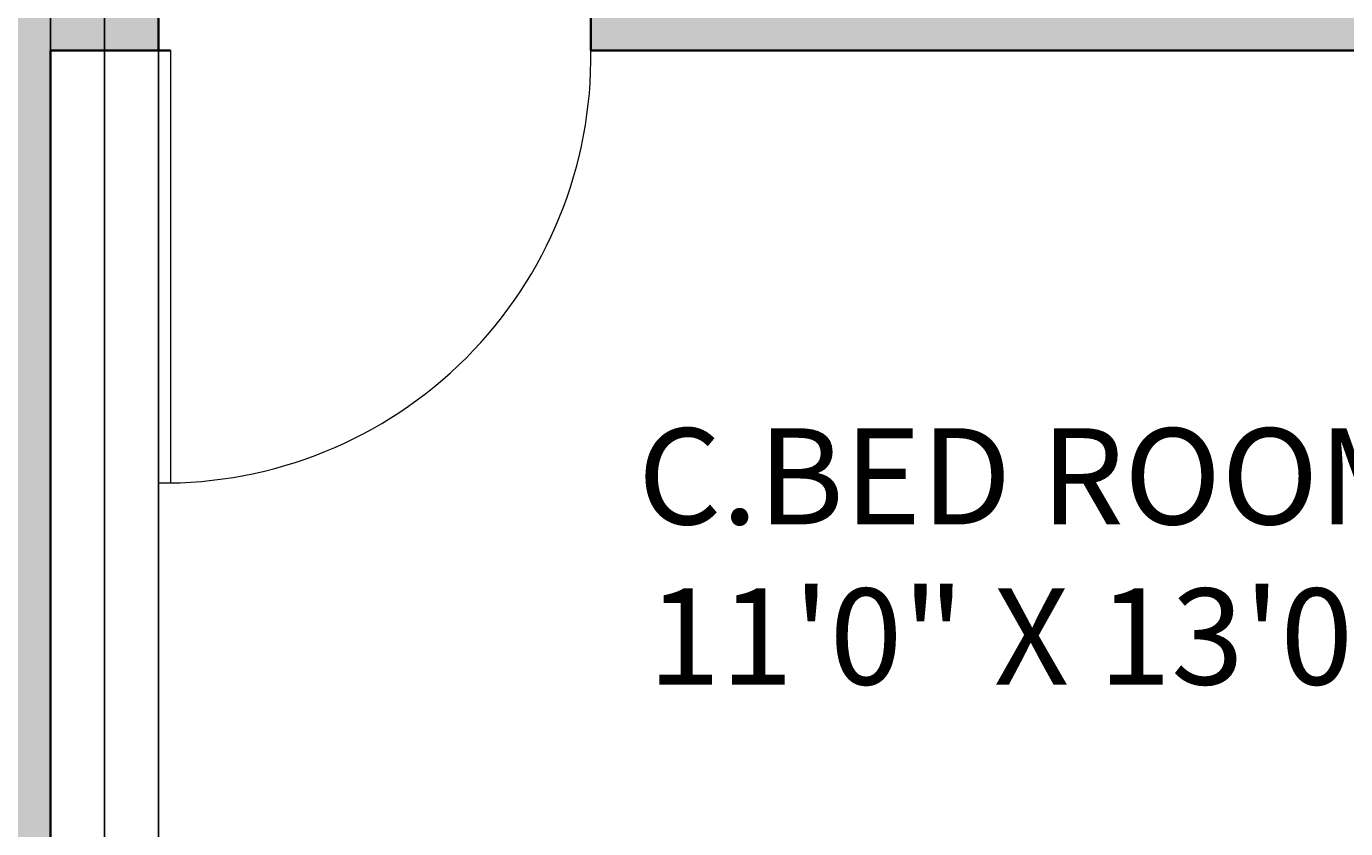
# Model space of a CAD drawing. Units: inches. Extents: x 1567 to 1964, y 1813 to 2447.
# Tile 5 of 28: x 1797 to 1907, y 2059 to 2125. Entities that reach past the tile are written whole.
import ezdxf

# ---------------------------------------------------------------- set-up
doc = ezdxf.new("R2010")
doc.units = ezdxf.units.IN
for name, color, linetype, lineweight in [('A-ANNO-DIMS', 2, 'Continuous', 18), ('A-AREA-IDEN', 7, 'Continuous', 18), ('A-DOOR', 4, 'Continuous', 18), ('A-WALL', 7, 'Continuous', 35)]:
    doc.layers.add(name, color=color, linetype=linetype, lineweight=lineweight)
doc.layers.add('A-FURN-PATT', color=252, linetype='Continuous', lineweight=13, true_color=0x939598)
doc.layers.add('A-WALL-PATT', color=251, linetype='Continuous', lineweight=13, true_color=0x636466)
doc.styles.get("Standard").update_dxf_attribs({"font": 'arial.ttf'})
doc.dimstyles.get("Standard").update_dxf_attribs({"dimtxt": 0.18, "dimasz": 0.18, "dimexe": 0.18, "dimexo": 0.0625, "dimgap": 0.09, "dimtad": 0, "dimtih": 1, "dimtoh": 1, "dimdec": 4, "dimzin": 0, "dimdsep": 46, "dimtxsty": 'Standard', "dimcen": 0.09, "dimadec": 0, "dimazin": 0, "dimtfac": 1, "dimtdec": 4, "dimtofl": 0, "dimtmove": 0, "dimatfit": 3, "dimfxl": 1, "dimtolj": 1, "dimtzin": 0, "dimarcsym": 0})

# ---------------------------------------------------------------- blocks, each defined once
blk = doc.blocks.new('DOOR-SWING-36IN')
for p, q in [((0, 36), (0, 0)), ((1, 36), (1, 0))]:
    blk.add_line(p, q)
blk.add_arc((0.5, 35.5), 35.5, 269.1931, 0.8069)
blk = doc.blocks.new('*D55')
at = {"layer": 'A-ANNO-DIMS', "color": 0, "lineweight": -2, "transparency": 16777216}
for p, q in [((1795.43, 1964.35), (1795.43, 2447.12)), ((1799.43, 1967.35), (1799.43, 2447.12)), ((1795.61, 2446.94), (1797.28, 2446.94)), ((1799.25, 2446.94), (1797.58, 2446.94))]:
    blk.add_line(p, q, dxfattribs=at)
at = {"layer": 'A-ANNO-DIMS', "color": 0, "transparency": 16777216}
for points in [[(1795.61, 2446.97), (1795.61, 2446.91), (1795.43, 2446.94)], [(1799.25, 2446.97), (1799.25, 2446.91), (1799.43, 2446.94)]]:
    blk.add_solid(points, dxfattribs=at)
at = {"layer": 'Defpoints', "color": 0, "transparency": 16777216}
for p in [(1799.43, 2446.94), (1799.43, 1967.29), (1795.43, 1964.29)]:
    blk.add_point(p, dxfattribs=at)
at = {"layer": 'A-ANNO-DIMS', "color": 0, "transparency": 16777216, "insert": (1797.43, 2446.94), "char_height": 0.18, "attachment_point": 5}
blk.add_mtext('\\A1;4', dxfattribs=at)
blk = doc.blocks.new('*D69')
at = {"layer": 'A-ANNO-DIMS', "color": 0, "lineweight": -2, "transparency": 16777216}
for p, q in [((1799.43, 2123.23), (1799.43, 1813.46)), ((1808.43, 2123.23), (1808.43, 1813.46)), ((1799.61, 1813.64), (1803.78, 1813.64)), ((1808.25, 1813.64), (1804.08, 1813.64))]:
    blk.add_line(p, q, dxfattribs=at)
at = {"layer": 'A-ANNO-DIMS', "color": 0, "transparency": 16777216}
for points in [[(1799.61, 1813.67), (1799.61, 1813.61), (1799.43, 1813.64)], [(1808.25, 1813.67), (1808.25, 1813.61), (1808.43, 1813.64)]]:
    blk.add_solid(points, dxfattribs=at)
at = {"layer": 'Defpoints', "color": 0, "transparency": 16777216}
for p in [(1799.43, 2123.29), (1808.43, 2123.29), (1808.43, 1813.64)]:
    blk.add_point(p, dxfattribs=at)
at = {"layer": 'A-ANNO-DIMS', "color": 0, "transparency": 16777216, "insert": (1803.93, 1813.64), "char_height": 0.18, "attachment_point": 5}
blk.add_mtext('\\A1;9', dxfattribs=at)
blk = doc.blocks.new('*D70')
at = {"layer": 'A-ANNO-DIMS', "color": 0, "lineweight": -2, "transparency": 16777216}
for p, q in [((1799.43, 1967.35), (1799.43, 2447.12)), ((1803.93, 1967.35), (1803.93, 2447.12)), ((1799.61, 2446.94), (1801.42, 2446.94)), ((1803.75, 2446.94), (1801.94, 2446.94))]:
    blk.add_line(p, q, dxfattribs=at)
at = {"layer": 'A-ANNO-DIMS', "color": 0, "transparency": 16777216}
for points in [[(1799.61, 2446.97), (1799.61, 2446.91), (1799.43, 2446.94)], [(1803.75, 2446.97), (1803.75, 2446.91), (1803.93, 2446.94)]]:
    blk.add_solid(points, dxfattribs=at)
at = {"layer": 'Defpoints', "color": 0, "transparency": 16777216}
for p in [(1803.93, 2446.94), (1799.43, 1967.29), (1803.93, 1967.29)]:
    blk.add_point(p, dxfattribs=at)
at = {"layer": 'A-ANNO-DIMS', "color": 0, "transparency": 16777216, "insert": (1801.68, 2446.94), "char_height": 0.18, "attachment_point": 5}
blk.add_mtext('\\A1;4.5', dxfattribs=at)
blk = doc.blocks.new('*D71')
at = {"layer": 'A-ANNO-DIMS', "color": 0, "lineweight": -2, "transparency": 16777216}
for p, q in [((1799.43, 1910.75), (1799.43, 2447.12)), ((1924.43, 1910.75), (1924.43, 2447.12)), ((1799.61, 2446.94), (1861.65, 2446.94)), ((1924.25, 2446.94), (1862.21, 2446.94))]:
    blk.add_line(p, q, dxfattribs=at)
at = {"layer": 'A-ANNO-DIMS', "color": 0, "transparency": 16777216}
for points in [[(1799.61, 2446.97), (1799.61, 2446.91), (1799.43, 2446.94)], [(1924.25, 2446.97), (1924.25, 2446.91), (1924.43, 2446.94)]]:
    blk.add_solid(points, dxfattribs=at)
at = {"layer": 'Defpoints', "color": 0, "transparency": 16777216}
for p in [(1924.43, 2446.94), (1799.43, 1910.69), (1924.43, 1910.69)]:
    blk.add_point(p, dxfattribs=at)
at = {"layer": 'A-ANNO-DIMS', "color": 0, "transparency": 16777216, "insert": (1861.93, 2446.94), "char_height": 0.18, "attachment_point": 5}
blk.add_mtext('\\A1;125', dxfattribs=at)

msp = doc.modelspace()

# ---------------------------------------------------------------- hatches: boundary and pattern name
at = {"layer": 'A-FURN-PATT'}
h = msp.add_hatch(color=256, dxfattribs=at)
h.dxf.hatch_style = 1
h.paths.add_polyline_path([(1697.3402, 2374.8316), (1682.1402, 2374.8316), (1682.1402, 2387.6316), (1637.3402, 2387.6316), (1637.3402, 2324.4315), (1697.3402, 2324.4315)])
h.paths.add_polyline_path([(1891.1093, 2375.8204), (1875.9094, 2375.8204), (1875.9094, 2388.6204), (1831.1094, 2388.6204), (1831.1094, 2325.4204), (1891.1093, 2325.4204)])
h.paths.add_polyline_path([(1702.5611, 2206.8057), (1702.5611, 2210.8057), (1699.7395, 2209.9436), (1697.013, 2209.2403), (1694.3857, 2208.6763), (1691.8615, 2208.2326), (1689.4443, 2207.8896), (1687.1381, 2207.6282), (1684.9469, 2207.4289), (1682.8747, 2207.2725), (1680.9233, 2207.1425), (1679.0865, 2207.0339), (1677.3558, 2206.9445), (1675.7229, 2206.8719), (1674.1794, 2206.8141), (1672.7169, 2206.7688), (1671.327, 2206.7339), (1670.0014, 2206.707), (1668.7314, 2206.6866), (1667.5072, 2206.6732), (1666.3188, 2206.668), (1665.1561, 2206.6722), (1664.009, 2206.6869), (1662.8675, 2206.7133), (1661.7215, 2206.7525), (1660.5611, 2206.8057), (1660.5611, 2202.8057), (1661.9932, 2202.9556), (1663.3314, 2203.0744), (1664.5899, 2203.1671), (1665.7831, 2203.2385), (1666.9254, 2203.2935), (1668.0311, 2203.3368), (1669.1145, 2203.3734), (1670.1902, 2203.4081), (1671.2724, 2203.4451), (1672.3759, 2203.4866), (1673.5155, 2203.534), (1674.706, 2203.5887), (1675.9621, 2203.6523), (1677.2986, 2203.7262), (1678.7304, 2203.8118), (1680.2722, 2203.9108), (1681.947, 2204.0272), (1683.8108, 2204.1769), (1685.9279, 2204.3782), (1688.3626, 2204.6496), (1691.179, 2205.0096), (1694.4413, 2205.4767), (1698.214, 2206.0692)])
h.paths.add_polyline_path([(1702.5611, 2218.8057), (1701.9821, 2217.9383), (1701.3316, 2217.191), (1700.6091, 2216.5515), (1699.8141, 2216.0071), (1698.946, 2215.5454), (1698.0041, 2215.1536), (1696.9879, 2214.8194), (1695.8969, 2214.5301), (1694.7328, 2214.2753), (1693.5072, 2214.0522), (1692.2339, 2213.8602), (1690.9266, 2213.6989), (1689.5994, 2213.5675), (1688.266, 2213.4654), (1686.9402, 2213.392), (1685.636, 2213.3467), (1684.3619, 2213.3287), (1683.1053, 2213.3361), (1681.8482, 2213.3668), (1680.5727, 2213.4187), (1679.2608, 2213.4898), (1677.8948, 2213.5779), (1676.4565, 2213.6811), (1674.9282, 2213.7971), (1673.2982, 2213.9236), (1671.5804, 2214.0573), (1669.795, 2214.1945), (1667.9622, 2214.3316), (1666.1022, 2214.4649), (1664.2352, 2214.5908), (1662.3814, 2214.7056), (1660.5611, 2214.8057), (1660.5611, 2206.8057), (1661.7215, 2206.7525), (1662.8675, 2206.7133), (1664.009, 2206.6869), (1665.1561, 2206.6722), (1666.3188, 2206.668), (1667.5072, 2206.6732), (1668.7314, 2206.6866), (1670.0014, 2206.707), (1671.327, 2206.7339), (1672.7169, 2206.7688), (1674.1794, 2206.8141), (1675.7229, 2206.8719), (1677.3558, 2206.9445), (1679.0865, 2207.0339), (1680.9233, 2207.1425), (1682.8747, 2207.2725), (1684.9469, 2207.4289), (1687.1381, 2207.6282), (1689.4443, 2207.8896), (1691.8615, 2208.2326), (1694.3857, 2208.6763), (1697.013, 2209.2403), (1699.7395, 2209.9436), (1702.5611, 2210.8057)])
h.paths.add_polyline_path([(1700.6091, 2216.5515), (1701.3316, 2217.191), (1701.9821, 2217.9383), (1702.5611, 2218.8057), (1702.5611, 2222.8057), (1689.452, 2222.8057), (1689.0171, 2222.4556), (1688.4521, 2222.0354), (1687.7806, 2221.5662), (1687.0235, 2221.067), (1686.2019, 2220.5566), (1685.3367, 2220.0541), (1684.4491, 2219.5785), (1683.56, 2219.1486), (1682.6867, 2218.7795), (1681.8312, 2218.4692), (1680.9918, 2218.212), (1680.1667, 2218.0019), (1679.3541, 2217.833), (1678.5524, 2217.6995), (1677.7597, 2217.5954), (1676.9744, 2217.5149), (1676.1942, 2217.4531), (1675.4146, 2217.4093), (1674.6309, 2217.384), (1673.8381, 2217.3774), (1673.0313, 2217.39), (1672.2056, 2217.4221), (1671.3562, 2217.4741), (1670.4782, 2217.5463), (1669.5642, 2217.639), (1668.5968, 2217.7516), (1667.5562, 2217.8833), (1666.4226, 2218.0336), (1665.1761, 2218.2017), (1663.7969, 2218.3869), (1662.2651, 2218.5885), (1660.5611, 2218.8057), (1660.5611, 2214.8057), (1662.3814, 2214.7056), (1664.2352, 2214.5908), (1666.1022, 2214.4649), (1667.9622, 2214.3316), (1669.795, 2214.1945), (1671.5804, 2214.0573), (1673.2982, 2213.9236), (1674.9282, 2213.7971), (1676.4565, 2213.6811), (1677.8948, 2213.5779), (1679.2608, 2213.4898), (1680.5727, 2213.4187), (1681.8482, 2213.3668), (1683.1053, 2213.3361), (1684.3619, 2213.3287), (1685.636, 2213.3467), (1686.9402, 2213.392), (1688.266, 2213.4654), (1689.5994, 2213.5675), (1690.9266, 2213.6989), (1692.2339, 2213.8602), (1693.5072, 2214.0522), (1694.7328, 2214.2753), (1695.8969, 2214.5301), (1696.9879, 2214.8194), (1698.0041, 2215.1536), (1698.946, 2215.5454), (1699.8141, 2216.0071)])
h.paths.add_polyline_path([(1687.0235, 2221.067), (1687.7806, 2221.5662), (1688.4521, 2222.0354), (1689.0171, 2222.4556), (1689.452, 2222.8057), (1660.5611, 2222.8057), (1660.5611, 2218.8057), (1662.2651, 2218.5885), (1663.7969, 2218.3869), (1665.1761, 2218.2017), (1666.4226, 2218.0336), (1667.5562, 2217.8833), (1668.5968, 2217.7516), (1669.5642, 2217.639), (1670.4782, 2217.5463), (1671.3562, 2217.4741), (1672.2056, 2217.4221), (1673.0313, 2217.39), (1673.8381, 2217.3774), (1674.6309, 2217.384), (1675.4146, 2217.4093), (1676.1942, 2217.4531), (1676.9744, 2217.5149), (1677.7597, 2217.5954), (1678.5524, 2217.6995), (1679.3541, 2217.833), (1680.1667, 2218.0019), (1680.9918, 2218.212), (1681.8312, 2218.4692), (1682.6867, 2218.7795), (1683.56, 2219.1486), (1684.4491, 2219.5785), (1685.3367, 2220.0541), (1686.2019, 2220.5566)], flags=17)
h.paths.add_polyline_path([(1702.5611, 2198.8057), (1698.9289, 2199.2412), (1695.8472, 2199.5774), (1693.2166, 2199.8257), (1690.9377, 2199.9973), (1688.9111, 2200.1033), (1687.0375, 2200.155), (1685.2174, 2200.1637), (1683.3514, 2200.1406), (1681.3514, 2200.0941), (1679.1736, 2200.0225), (1676.7858, 2199.921), (1674.1554, 2199.7852), (1671.2502, 2199.6103), (1668.0377, 2199.3919), (1664.4854, 2199.1252), (1660.5611, 2198.8057), (1660.5611, 2194.8057), (1662.2697, 2194.9771), (1663.9673, 2195.0999), (1665.6339, 2195.1809), (1667.2495, 2195.227), (1668.7941, 2195.2449), (1670.2478, 2195.2414), (1671.5906, 2195.2233), (1672.8026, 2195.1974), (1673.8739, 2195.1689), (1674.8359, 2195.1364), (1675.7302, 2195.0967), (1676.5982, 2195.0469), (1677.4817, 2194.9838), (1678.422, 2194.9043), (1679.4609, 2194.8055), (1680.6397, 2194.6842), (1682.005, 2194.5341), (1683.6223, 2194.335), (1685.562, 2194.0637), (1687.8945, 2193.6967), (1690.6902, 2193.2108), (1694.0196, 2192.5826), (1697.9531, 2191.7887), (1702.5611, 2190.8057)])
h.paths.add_polyline_path([(1702.5611, 2206.8057), (1698.214, 2206.0692), (1694.4413, 2205.4767), (1691.179, 2205.0096), (1688.3626, 2204.6496), (1685.9279, 2204.3782), (1683.8108, 2204.1769), (1681.947, 2204.0272), (1680.2722, 2203.9108), (1678.7304, 2203.8118), (1677.2986, 2203.7262), (1675.9621, 2203.6523), (1674.706, 2203.5887), (1673.5155, 2203.534), (1672.3759, 2203.4866), (1671.2724, 2203.4451), (1670.1902, 2203.4081), (1669.1145, 2203.3734), (1668.0311, 2203.3368), (1666.9254, 2203.2935), (1665.7831, 2203.2385), (1664.5899, 2203.1671), (1663.3314, 2203.0744), (1661.9932, 2202.9556), (1660.5611, 2202.8057), (1660.5611, 2198.8057), (1664.4854, 2199.1252), (1668.0377, 2199.3919), (1671.2502, 2199.6103), (1674.1554, 2199.7852), (1676.7858, 2199.921), (1679.1736, 2200.0225), (1681.3514, 2200.0941), (1683.3514, 2200.1406), (1685.2174, 2200.1637), (1687.0375, 2200.155), (1688.9111, 2200.1033), (1690.9377, 2199.9973), (1693.2166, 2199.8257), (1695.8472, 2199.5774), (1698.9289, 2199.2412), (1702.5611, 2198.8057)])
h.paths.add_polyline_path([(1702.5611, 2190.8057), (1697.9531, 2191.7887), (1694.0196, 2192.5826), (1690.6902, 2193.2108), (1687.8945, 2193.6967), (1685.562, 2194.0637), (1683.6223, 2194.335), (1682.005, 2194.5341), (1680.6397, 2194.6842), (1679.4609, 2194.8055), (1678.422, 2194.9043), (1677.4817, 2194.9838), (1676.5982, 2195.0469), (1675.7302, 2195.0967), (1674.8359, 2195.1364), (1673.8739, 2195.1689), (1672.8026, 2195.1974), (1671.5906, 2195.2233), (1670.2478, 2195.2414), (1668.7941, 2195.2449), (1667.2495, 2195.227), (1665.6339, 2195.1809), (1663.9673, 2195.0999), (1662.2697, 2194.9771), (1660.5611, 2194.8057), (1660.5611, 2190.8057), (1665.9637, 2190.2699), (1670.5105, 2189.7867), (1674.3035, 2189.3504), (1677.4445, 2188.9552), (1680.0354, 2188.5951), (1682.1782, 2188.2644), (1683.9747, 2187.9571), (1685.5268, 2187.6675), (1686.9225, 2187.3901), (1688.1943, 2187.1216), (1689.3606, 2186.859), (1690.4399, 2186.5993), (1691.4508, 2186.3396), (1692.4118, 2186.0769), (1693.3413, 2185.8084), (1694.2579, 2185.531), (1695.1786, 2185.2422), (1696.1142, 2184.9406), (1697.0739, 2184.6252), (1698.0671, 2184.2949), (1699.1032, 2183.9489), (1700.1913, 2183.586), (1701.3408, 2183.2053), (1702.5611, 2182.8057)])
h.paths.add_polyline_path([(1702.5611, 2182.8057), (1701.3408, 2183.2053), (1700.1913, 2183.586), (1699.1032, 2183.9489), (1698.0671, 2184.2949), (1697.0739, 2184.6252), (1696.1142, 2184.9406), (1695.1786, 2185.2422), (1694.2579, 2185.531), (1693.3413, 2185.8084), (1692.4118, 2186.0769), (1691.4508, 2186.3396), (1690.4399, 2186.5993), (1689.3606, 2186.859), (1688.1943, 2187.1216), (1686.9225, 2187.3901), (1685.5268, 2187.6675), (1683.9747, 2187.9571), (1682.1782, 2188.2644), (1680.0354, 2188.5951), (1677.4445, 2188.9552), (1674.3035, 2189.3504), (1670.5105, 2189.7867), (1665.9637, 2190.2699), (1660.5611, 2190.8057), (1660.5611, 2186.8057), (1663.5709, 2186.52), (1666.0965, 2186.2414), (1668.1979, 2185.9698), (1669.9351, 2185.7048), (1671.3681, 2185.446), (1672.5568, 2185.1931), (1673.5613, 2184.9458), (1674.4415, 2184.7037), (1675.2485, 2184.4664), (1675.9976, 2184.2328), (1677.0295, 2183.8907), (1678.2492, 2183.4332), (1679.354, 2182.9669), (1680.4123, 2182.4724), (1681.3757, 2181.9718), (1682.2435, 2181.4594), (1683.1864, 2180.8057), (1702.5611, 2180.8057)])
h.paths.add_polyline_path([(1677.3469, 2183.7716), (1676.6949, 2184.0016), (1675.9976, 2184.2328), (1675.2485, 2184.4664), (1674.4415, 2184.7037), (1673.5613, 2184.9458), (1672.5568, 2185.1931), (1671.3681, 2185.446), (1669.9351, 2185.7048), (1668.1979, 2185.9698), (1666.0965, 2186.2414), (1663.5709, 2186.52), (1660.5611, 2186.8057), (1660.5611, 2180.8057), (1683.1506, 2180.8057), (1682.802, 2181.0722), (1682.4264, 2181.3326), (1682.0201, 2181.5913), (1681.586, 2181.8476), (1681.1268, 2182.1011), (1680.6453, 2182.3513), (1680.1443, 2182.5976), (1679.6266, 2182.8395), (1679.0933, 2183.0769), (1678.5398, 2183.3105), (1677.9598, 2183.5417)], flags=17)
h.paths.add_polyline_path([(1824.4511, 2199.9016), (1824.089, 2199.9302), (1824.0595, 2199.9372), (1824.0397, 2199.9406), (1823.5413, 2200.0576), (1823.4095, 2200.0864), (1823.0664, 2200.1559), (1822.6419, 2200.2361), (1822.1519, 2200.3222), (1821.6126, 2200.4093), (1821.0401, 2200.4925), (1820.4505, 2200.5669), (1819.8599, 2200.6276), (1819.2845, 2200.6697), (1818.7366, 2200.6896), (1818.2141, 2200.688), (1817.7112, 2200.6668), (1817.222, 2200.6281), (1816.7405, 2200.5737), (1816.261, 2200.5057), (1815.7776, 2200.4259), (1815.2845, 2200.3364), (1814.3007, 2200.149), (1813.3315, 2199.9765), (1812.406, 2199.8514), (1811.6868, 2199.7739), (1810.8992, 2199.7121), (1810.0345, 2199.6697), (1809.0854, 2199.6497), (1808.0514, 2199.6502), (1806.9334, 2199.6683), (1805.7324, 2199.701), (1804.4493, 2199.7454), (1803.0852, 2199.7986), (1801.641, 2199.8577), (1800.1178, 2199.9197), (1798.5134, 2199.9818), (1796.8144, 2200.0415), (1795.004, 2200.0962), (1793.0657, 2200.1437), (1790.9828, 2200.1814), (1788.7389, 2200.2068), (1786.3171, 2200.2177), (1783.7011, 2200.2114), (1780.8715, 2200.185), (1777.7988, 2200.1326), (1774.4506, 2200.0481), (1770.7948, 2199.9249), (1766.7992, 2199.7569), (1762.4316, 2199.5376), (1757.6596, 2199.2606), (1752.4511, 2198.9197), (1752.4511, 2193.4197), (1761.2668, 2193.6071), (1768.3671, 2193.7934), (1773.9821, 2193.9778), (1778.3417, 2194.1593), (1781.6759, 2194.3369), (1784.2148, 2194.5096), (1786.1882, 2194.6764), (1787.8261, 2194.8364), (1789.3219, 2194.9887), (1790.7226, 2195.1333), (1792.0383, 2195.27), (1793.2792, 2195.3989), (1794.4557, 2195.52), (1795.5781, 2195.6333), (1796.6564, 2195.7387), (1797.7011, 2195.8364), (1798.7216, 2195.9259), (1799.7245, 2196.0057), (1800.7158, 2196.0737), (1801.7011, 2196.1281), (1802.6865, 2196.1668), (1803.6777, 2196.188), (1804.6806, 2196.1896), (1805.7011, 2196.1697), (1806.7423, 2196.1273), (1807.7962, 2196.0643), (1808.852, 2195.9837), (1809.899, 2195.8885), (1810.9265, 2195.7815), (1811.9238, 2195.6658), (1812.88, 2195.5442), (1813.7845, 2195.4197), (1814.6296, 2195.2948), (1815.4205, 2195.1704), (1816.1656, 2195.0469), (1816.873, 2194.9249), (1817.5511, 2194.8049), (1818.2083, 2194.6873), (1818.8527, 2194.5726), (1819.4928, 2194.4614), (1820.1348, 2194.3554), (1820.7773, 2194.2615), (1821.4169, 2194.1882), (1822.0501, 2194.1437), (1822.6735, 2194.1363), (1823.2838, 2194.1743), (1823.8775, 2194.266), (1824.4511, 2194.4197)])
h.paths.add_polyline_path([(1821.4716, 2190.5098), (1820.4303, 2190.5708), (1819.3811, 2190.6415), (1818.3339, 2190.7186), (1817.2985, 2190.7986), (1816.2845, 2190.8781), (1815.2976, 2190.9542), (1814.3274, 2191.0259), (1813.3592, 2191.0927), (1812.3782, 2191.1541), (1811.3699, 2191.2097), (1810.3196, 2191.2589), (1809.2127, 2191.3013), (1808.0345, 2191.3364), (1806.7708, 2191.3634), (1805.4094, 2191.3807), (1803.9387, 2191.3862), (1802.3469, 2191.3781), (1800.6223, 2191.3543), (1798.7532, 2191.313), (1796.7278, 2191.2521), (1794.5344, 2191.1697), (1792.128, 2191.0648), (1789.33, 2190.9393), (1785.9285, 2190.7962), (1781.7115, 2190.6385), (1776.4672, 2190.469), (1769.9836, 2190.2908), (1762.0489, 2190.1067), (1752.4511, 2189.9197), (1752.4511, 2185.4197), (1758.363, 2185.5846), (1763.4179, 2185.7075), (1767.7199, 2185.7933), (1771.373, 2185.8468), (1774.4811, 2185.873), (1777.1484, 2185.8768), (1779.4787, 2185.8629), (1781.5761, 2185.8364), (1783.5287, 2185.8014), (1785.3606, 2185.7596), (1787.0802, 2185.7119), (1788.6959, 2185.6593), (1790.2158, 2185.6028), (1791.6484, 2185.5434), (1793.0018, 2185.4821), (1794.2844, 2185.4197), (1795.5065, 2185.3576), (1796.6861, 2185.298), (1797.8433, 2185.2432), (1798.998, 2185.1958), (1800.1703, 2185.1581), (1801.3801, 2185.1326), (1802.6476, 2185.1218), (1803.9928, 2185.1281), (1805.4444, 2185.1555), (1807.0663, 2185.2147), (1808.9315, 2185.3178), (1811.1126, 2185.477), (1813.6823, 2185.7046), (1816.7135, 2186.0128), (1820.2788, 2186.4138), (1824.4511, 2186.9197), (1824.4511, 2190.4197), (1823.4918, 2190.4309), (1822.4954, 2190.4621)])
h.paths.add_polyline_path([(1797.3762, 2216.0584), (1797.6199, 2216.2267), (1797.9558, 2216.3355), (1798.3017, 2216.3703), (1798.5761, 2216.3781), (1798.8974, 2216.3703), (1799.2714, 2216.3468), (1799.704, 2216.3078), (1800.2011, 2216.2531), (1800.7695, 2216.1829), (1801.4205, 2216.0981), (1802.1662, 2215.9996), (1803.0188, 2215.8885), (1803.9906, 2215.7656), (1805.0937, 2215.632), (1806.3404, 2215.4886), (1807.7428, 2215.3364), (1809.3101, 2215.1764), (1811.039, 2215.0096), (1812.9232, 2214.8369), (1814.9563, 2214.6593), (1817.132, 2214.4778), (1819.444, 2214.2934), (1821.8858, 2214.1071), (1824.4511, 2213.9197), (1824.4511, 2217.9197), (1752.4511, 2217.9197), (1752.4511, 2214.9197), (1757.2739, 2214.8973), (1761.6432, 2214.8338), (1765.5973, 2214.7352), (1769.1751, 2214.6072), (1772.4149, 2214.4559), (1775.3554, 2214.2869), (1778.0352, 2214.1063), (1780.4928, 2213.9197), (1782.7607, 2213.7329), (1784.8476, 2213.5499), (1786.7557, 2213.3748), (1788.4876, 2213.2114), (1790.0456, 2213.0636), (1791.4322, 2212.9354), (1792.6499, 2212.8305), (1793.7011, 2212.7531), (1794.5904, 2212.7059), (1795.3313, 2212.688), (1795.9394, 2212.6974), (1796.4303, 2212.7322), (1796.8196, 2212.7905), (1797.123, 2212.8703), (1797.356, 2212.9695), (1797.5344, 2213.0864), (1797.6716, 2213.2187), (1797.7727, 2213.3637), (1797.8406, 2213.5185), (1797.8782, 2213.6801), (1797.8884, 2213.8457), (1797.8743, 2214.0122), (1797.8386, 2214.1767), (1797.7844, 2214.3364), (1797.7149, 2214.4889), (1797.6347, 2214.6346), (1797.5486, 2214.7744), (1797.3327, 2215.109), (1797.178, 2215.4303), (1797.1896, 2215.7939)])
h.paths.add_polyline_path([(1804.7872, 2210.6789), (1804.546, 2211.022), (1804.3512, 2211.3917), (1804.2466, 2211.7546), (1804.2574, 2212.0998), (1804.4058, 2212.4178), (1804.7068, 2212.7007), (1805.1359, 2212.9124), (1805.5279, 2212.9926), (1805.8136, 2213.0154), (1806.1178, 2213.0031), (1806.4405, 2212.9529), (1806.7929, 2212.867), (1807.1893, 2212.7489), (1807.6438, 2212.602), (1808.1706, 2212.4297), (1808.7838, 2212.2355), (1809.4976, 2212.0227), (1810.3261, 2211.7947), (1811.2868, 2211.5533), (1812.4101, 2211.2928), (1813.7297, 2211.0059), (1815.2793, 2210.6854), (1817.0925, 2210.3238), (1819.2031, 2209.9139), (1821.6447, 2209.4483), (1824.4511, 2208.9197), (1824.4511, 2213.9197), (1821.8858, 2214.1071), (1819.444, 2214.2934), (1817.132, 2214.4778), (1814.9563, 2214.6593), (1812.9232, 2214.8369), (1811.039, 2215.0096), (1809.3101, 2215.1764), (1807.7428, 2215.3364), (1806.3404, 2215.4886), (1805.0937, 2215.632), (1803.9906, 2215.7656), (1803.0188, 2215.8885), (1802.1662, 2215.9996), (1801.4205, 2216.0981), (1800.7695, 2216.1829), (1800.2011, 2216.2531), (1799.704, 2216.3078), (1799.2714, 2216.3468), (1798.8974, 2216.3703), (1798.5761, 2216.3781), (1798.3017, 2216.3703), (1798.0683, 2216.3468), (1797.87, 2216.3078), (1797.7011, 2216.2531), (1797.5566, 2216.1831), (1797.4355, 2216.0994), (1797.3378, 2216.004), (1797.2636, 2215.8989), (1797.2128, 2215.7859), (1797.1855, 2215.6671), (1797.1816, 2215.5444), (1797.2011, 2215.4197), (1797.2433, 2215.2946), (1797.304, 2215.1684), (1797.3783, 2215.0403), (1797.4615, 2214.9093), (1797.6718, 2214.5836), (1797.8218, 2214.2545), (1797.8933, 2213.9247), (1797.8728, 2213.5918), (1797.7366, 2213.2814), (1797.4586, 2213.0132), (1797.123, 2212.8703), (1796.8196, 2212.7905), (1796.4303, 2212.7322), (1795.9394, 2212.6974), (1795.3313, 2212.688), (1794.5904, 2212.7059), (1793.7011, 2212.7531), (1792.6499, 2212.8305), (1791.4322, 2212.9354), (1790.0456, 2213.0636), (1788.4876, 2213.2114), (1786.7557, 2213.3748), (1784.8476, 2213.5499), (1782.7607, 2213.7329), (1780.4928, 2213.9197), (1778.0352, 2214.1063), (1775.3554, 2214.2869), (1772.4149, 2214.4559), (1769.1751, 2214.6072), (1765.5973, 2214.7352), (1761.6432, 2214.8338), (1757.2739, 2214.8973), (1752.4511, 2214.9197), (1752.4511, 2209.9197), (1759.4745, 2210.0625), (1765.2786, 2210.1242), (1770.027, 2210.1175), (1773.8834, 2210.0551), (1777.0112, 2209.9498), (1779.5741, 2209.8143), (1781.7357, 2209.6611), (1783.6594, 2209.5031), (1785.4813, 2209.3506), (1787.2265, 2209.2049), (1788.8926, 2209.0651), (1790.4771, 2208.9301), (1791.9777, 2208.7991), (1793.3919, 2208.671), (1794.7171, 2208.5449), (1795.9511, 2208.4197), (1797.0922, 2208.2952), (1798.1425, 2208.1736), (1799.1049, 2208.0579), (1799.9823, 2207.951), (1800.7778, 2207.8558), (1801.4941, 2207.7752), (1802.1342, 2207.7122), (1802.7011, 2207.6697), (1803.1982, 2207.65), (1803.6308, 2207.6528), (1804.0048, 2207.6771), (1804.3261, 2207.7218), (1804.6005, 2207.7861), (1804.8339, 2207.869), (1805.0322, 2207.9694), (1805.2011, 2208.0864), (1805.3455, 2208.2189), (1805.4654, 2208.365), (1805.56, 2208.5229), (1805.6282, 2208.6906), (1805.6691, 2208.866), (1805.6816, 2209.0473), (1805.6648, 2209.2326), (1805.6178, 2209.4197), (1805.5406, 2209.6072), (1805.4381, 2209.7947), (1805.316, 2209.9822), (1805.1803, 2210.1697), (1805.0367, 2210.3572)])
h.paths.add_polyline_path([(1801.4941, 2207.7752), (1800.7778, 2207.8558), (1799.9823, 2207.951), (1799.1049, 2208.0579), (1798.1425, 2208.1736), (1797.0922, 2208.2952), (1795.9511, 2208.4197), (1794.7171, 2208.5449), (1793.3919, 2208.671), (1791.9777, 2208.7991), (1790.4771, 2208.9301), (1788.8926, 2209.0651), (1787.2265, 2209.2049), (1785.4813, 2209.3506), (1783.6594, 2209.5031), (1781.7357, 2209.6611), (1779.5741, 2209.8143), (1777.0112, 2209.9498), (1773.8834, 2210.0551), (1770.027, 2210.1175), (1765.2786, 2210.1242), (1759.4745, 2210.0625), (1752.4511, 2209.9197), (1752.4511, 2205.4197), (1757.7354, 2205.2545), (1762.3821, 2205.1294), (1766.4565, 2205.0374), (1770.024, 2204.9718), (1773.1502, 2204.9258), (1775.9003, 2204.8924), (1778.3399, 2204.8649), (1780.5344, 2204.8364), (1782.5421, 2204.8014), (1784.3925, 2204.7596), (1786.1082, 2204.7119), (1787.7115, 2204.6593), (1789.225, 2204.6028), (1790.6711, 2204.5434), (1792.0724, 2204.4821), (1793.4511, 2204.4197), (1794.8241, 2204.3576), (1796.1855, 2204.2973), (1797.5234, 2204.241), (1798.8261, 2204.1906), (1800.082, 2204.1479), (1801.2792, 2204.115), (1802.4062, 2204.0939), (1803.4511, 2204.0864), (1804.4051, 2204.0942), (1805.2701, 2204.1176), (1806.0512, 2204.1567), (1806.7532, 2204.2114), (1807.381, 2204.2817), (1807.9394, 2204.3676), (1808.4334, 2204.4692), (1808.8678, 2204.5864), (1809.248, 2204.7187), (1809.5813, 2204.8637), (1809.8756, 2205.0185), (1810.1386, 2205.1801), (1810.3782, 2205.3457), (1810.6022, 2205.5122), (1810.9725, 2205.7941), (1811.3803, 2206.072), (1811.739, 2206.2612), (1812.0032, 2206.3781), (1812.2869, 2206.4793), (1812.5931, 2206.563), (1812.9246, 2206.6271), (1813.2845, 2206.6697), (1813.6746, 2206.6894), (1814.0931, 2206.6867), (1814.5369, 2206.6624), (1815.0032, 2206.6176), (1815.489, 2206.5534), (1815.9915, 2206.4705), (1816.5076, 2206.3701), (1817.0345, 2206.2531), (1817.5753, 2206.1196), (1818.1582, 2205.9666), (1818.8172, 2205.7902), (1819.5865, 2205.5864), (1820.5004, 2205.3514), (1821.5931, 2205.0812), (1822.8986, 2204.7719), (1824.4511, 2204.4197), (1824.4511, 2208.9197), (1821.6447, 2209.4483), (1819.2031, 2209.9139), (1817.0925, 2210.3238), (1815.2793, 2210.6854), (1813.7297, 2211.0059), (1812.4101, 2211.2928), (1811.2868, 2211.5533), (1810.3261, 2211.7947), (1809.4976, 2212.0227), (1808.7838, 2212.2355), (1808.1706, 2212.4297), (1807.6438, 2212.602), (1807.1893, 2212.7489), (1806.7929, 2212.867), (1806.4405, 2212.9529), (1806.1178, 2213.0031), (1805.8136, 2213.0154), (1805.5279, 2212.9926), (1805.2638, 2212.9386), (1805.024, 2212.8572), (1804.8116, 2212.7524), (1804.6295, 2212.6281), (1804.4806, 2212.4881), (1804.3678, 2212.3364), (1804.2931, 2212.1764), (1804.2545, 2212.0096), (1804.2491, 2211.8369), (1804.274, 2211.6593), (1804.3263, 2211.4778), (1804.4029, 2211.2934), (1804.5011, 2211.1071), (1804.6178, 2210.9197), (1804.7496, 2210.7322), (1804.8912, 2210.5447), (1805.154, 2210.2061), (1805.3962, 2209.8715), (1805.5964, 2209.5053), (1805.688, 2209.1402), (1805.6629, 2208.7758), (1805.5257, 2208.4385), (1805.2839, 2208.1437), (1804.9434, 2207.9078), (1804.6005, 2207.7861), (1804.3261, 2207.7218), (1804.0048, 2207.6771), (1803.6308, 2207.6528), (1803.1982, 2207.65), (1802.7011, 2207.6697), (1802.1342, 2207.7122)])
h.paths.add_polyline_path([(1824.4511, 2204.4197), (1822.8986, 2204.7719), (1821.5931, 2205.0812), (1820.5004, 2205.3514), (1819.5865, 2205.5864), (1818.8172, 2205.7902), (1818.1582, 2205.9666), (1817.5753, 2206.1196), (1817.0345, 2206.2531), (1816.5076, 2206.3701), (1815.9915, 2206.4705), (1815.489, 2206.5534), (1815.0032, 2206.6176), (1814.5369, 2206.6624), (1814.0931, 2206.6867), (1813.6746, 2206.6894), (1813.2845, 2206.6697), (1812.9246, 2206.6271), (1812.5931, 2206.563), (1812.2869, 2206.4793), (1812.0032, 2206.3781), (1811.739, 2206.2612), (1811.4915, 2206.1307), (1811.2576, 2205.9884), (1811.0345, 2205.8364), (1810.8183, 2205.6767), (1810.4357, 2205.3854), (1810.1386, 2205.1801), (1809.8756, 2205.0185), (1809.5813, 2204.8637), (1809.248, 2204.7187), (1808.8678, 2204.5864), (1808.4334, 2204.4692), (1807.9394, 2204.3676), (1807.381, 2204.2817), (1806.7532, 2204.2114), (1806.0512, 2204.1567), (1805.2701, 2204.1176), (1804.4051, 2204.0942), (1803.4511, 2204.0864), (1802.4062, 2204.0939), (1801.2792, 2204.115), (1800.082, 2204.1479), (1798.8261, 2204.1906), (1797.5234, 2204.241), (1796.1855, 2204.2973), (1794.8241, 2204.3576), (1793.4511, 2204.4197), (1792.0724, 2204.4821), (1790.6711, 2204.5434), (1789.225, 2204.6028), (1787.7115, 2204.6593), (1786.1082, 2204.7119), (1784.3925, 2204.7596), (1782.5421, 2204.8014), (1780.5344, 2204.8364), (1778.3399, 2204.8649), (1775.9003, 2204.8924), (1773.1502, 2204.9258), (1770.024, 2204.9718), (1766.4565, 2205.0374), (1762.3821, 2205.1294), (1757.7354, 2205.2545), (1752.4511, 2205.4197), (1752.4511, 2198.9197), (1757.6596, 2199.2606), (1762.4316, 2199.5376), (1766.7992, 2199.7569), (1770.7948, 2199.9249), (1774.4506, 2200.0481), (1777.7988, 2200.1326), (1780.8715, 2200.185), (1783.7011, 2200.2114), (1786.3171, 2200.2177), (1788.7389, 2200.2068), (1790.9828, 2200.1814), (1793.0657, 2200.1437), (1795.004, 2200.0962), (1796.8144, 2200.0415), (1798.5134, 2199.9818), (1800.1178, 2199.9197), (1801.641, 2199.8577), (1803.0852, 2199.7986), (1804.4493, 2199.7454), (1805.7324, 2199.701), (1806.9334, 2199.6683), (1808.0514, 2199.6502), (1809.0854, 2199.6497), (1810.0345, 2199.6697), (1810.8992, 2199.7121), (1811.6868, 2199.7739), (1812.406, 2199.8514), (1813.0657, 2199.9406), (1813.6746, 2200.0376), (1814.2415, 2200.1385), (1814.7752, 2200.2394), (1815.2845, 2200.3364), (1815.7776, 2200.4259), (1816.261, 2200.5057), (1816.7405, 2200.5737), (1817.222, 2200.6281), (1817.7112, 2200.6668), (1818.2141, 2200.688), (1818.7366, 2200.6896), (1819.2845, 2200.6697), (1819.8599, 2200.6276), (1820.4505, 2200.5669), (1821.0401, 2200.4925), (1821.6126, 2200.4093), (1822.1519, 2200.3222), (1822.6419, 2200.2361), (1823.0664, 2200.1559), (1823.5408, 2200.0598), (1824.0595, 2199.9372), (1824.1105, 2199.9285), (1824.1888, 2199.9223), (1824.2953, 2199.9201), (1824.4511, 2199.9197)])
h.paths.add_polyline_path([(1795.4295, 2021.5492), (1771.4295, 2021.5492), (1771.4295, 1988.29), (1735.4295, 1988.29), (1735.4295, 2055.79), (1711.4295, 2055.79), (1711.4295, 1964.29), (1795.4295, 1964.29)])
h.paths.add_polyline_path([(1681.4295, 2063.29), (1674.0411, 2043.4455), (1681.4295, 2043.4455), (1688.818, 2043.4455)])
h.paths.add_polyline_path([(1843.2327, 2065.967), (1919.26, 2065.967), (1919.26, 2095.8187), (1843.2327, 2095.8187)], flags=9)
h = msp.add_hatch(color=256, dxfattribs=at)
h.dxf.hatch_style = 1
h.paths.add_polyline_path([(1642.2233, 2241.7446), (1623.1648, 2241.9976), (1622.8462, 2217.9997), (1641.9047, 2217.7467)])
h.paths.add_polyline_path([(1641.9047, 2217.7467), (1622.8462, 2217.9997), (1622.5277, 2194.0018), (1641.5862, 2193.7488)])
h.paths.add_polyline_path([(1641.5862, 2193.7488), (1622.5277, 2194.0018), (1622.2091, 2170.0039), (1641.2677, 2169.7509)])
h.paths.add_polyline_path([(1671.2154, 2243.8726, -0.23606798), (1673.5306, 2245.0302), (1673.5306, 2246.1879), (1653.8509, 2246.1879), (1653.8509, 2245.0302, -0.23606798), (1656.1662, 2243.8726), (1656.1662, 2233.4539, -0.23606798), (1653.8509, 2232.2963), (1653.8509, 2231.1387, 0.11764706), (1673.5306, 2231.1387), (1673.5306, 2232.2963, -0.23606798), (1671.2154, 2233.4539)])
h.paths.add_polyline_path([(1703.7736, 2243.8726, -0.23606798), (1706.0889, 2245.0302), (1706.0889, 2246.1879), (1686.4092, 2246.1879), (1686.4092, 2245.0302, -0.23606798), (1688.7245, 2243.8726), (1688.7245, 2233.4539, -0.23606798), (1686.4092, 2232.2963), (1686.4092, 2231.1387, 0.11764706), (1706.0889, 2231.1387), (1706.0889, 2232.2963, -0.23606798), (1703.7736, 2233.4539)])
h.paths.add_polyline_path([(1782.6855, 2225.9197), (1766.2168, 2225.9197), (1764.9668, 2217.9197), (1783.9356, 2217.9197)])
h.paths.add_polyline_path([(1810.6855, 2225.9197), (1794.2168, 2225.9197), (1792.9668, 2217.9197), (1811.9356, 2217.9197)])
h.paths.add_polyline_path([(1752.4511, 2209.4041), (1744.4511, 2208.1541), (1744.4511, 2191.6853), (1752.4511, 2190.4354)])
h.paths.add_polyline_path([(1783.9356, 2181.9197), (1764.9668, 2181.9197), (1766.2168, 2173.9197), (1782.6855, 2173.9197)])
h.paths.add_polyline_path([(1811.9356, 2181.9197), (1792.9668, 2181.9197), (1794.2168, 2173.9197), (1810.6855, 2173.9197)])
h.paths.add_polyline_path([(1832.4511, 2208.1541), (1824.4511, 2209.4041), (1824.4511, 2190.4354), (1832.4511, 2191.6853)])
h.paths.add_polyline_path([(1824.4511, 2194.4197), (1823.8775, 2194.266), (1823.2838, 2194.1743), (1822.6735, 2194.1363), (1822.0501, 2194.1437), (1821.4169, 2194.1882), (1820.7773, 2194.2615), (1820.1348, 2194.3554), (1819.4928, 2194.4614), (1818.8527, 2194.5726), (1818.2083, 2194.6873), (1817.5511, 2194.8049), (1816.873, 2194.9249), (1816.1656, 2195.0469), (1815.4205, 2195.1704), (1814.6296, 2195.2948), (1813.7845, 2195.4197), (1812.88, 2195.5442), (1811.9238, 2195.6658), (1810.9265, 2195.7815), (1809.899, 2195.8885), (1808.852, 2195.9837), (1807.7962, 2196.0643), (1806.7423, 2196.1273), (1805.7011, 2196.1697), (1804.6806, 2196.1896), (1803.6777, 2196.188), (1802.6865, 2196.1668), (1801.7011, 2196.1281), (1800.7158, 2196.0737), (1799.7245, 2196.0057), (1798.7216, 2195.9259), (1797.7011, 2195.8364), (1796.6564, 2195.7387), (1795.5781, 2195.6333), (1794.4557, 2195.52), (1793.2792, 2195.3989), (1792.0383, 2195.27), (1790.7226, 2195.1333), (1789.3219, 2194.9887), (1787.8261, 2194.8364), (1786.1882, 2194.6764), (1784.2148, 2194.5096), (1781.6759, 2194.3369), (1778.3417, 2194.1593), (1773.9821, 2193.9778), (1768.3671, 2193.7934), (1761.2668, 2193.6071), (1752.4511, 2193.4197), (1752.4511, 2189.9197), (1762.0489, 2190.1067), (1769.9836, 2190.2908), (1776.4672, 2190.469), (1781.7115, 2190.6385), (1785.9285, 2190.7962), (1789.33, 2190.9393), (1792.128, 2191.0648), (1794.5344, 2191.1697), (1796.7278, 2191.2521), (1798.7532, 2191.313), (1800.6223, 2191.3543), (1802.3469, 2191.3781), (1803.9387, 2191.3862), (1805.4094, 2191.3807), (1806.7708, 2191.3634), (1808.0345, 2191.3364), (1809.2127, 2191.3013), (1810.3196, 2191.2589), (1811.3699, 2191.2097), (1812.3782, 2191.1541), (1813.3592, 2191.0927), (1814.3274, 2191.0259), (1815.2976, 2190.9542), (1816.2845, 2190.8781), (1817.2985, 2190.7986), (1818.3339, 2190.7186), (1819.3811, 2190.6415), (1820.4303, 2190.5708), (1821.4716, 2190.5098), (1822.4954, 2190.4621), (1823.4918, 2190.4309), (1824.3581, 2190.4208), (1824.4511, 2190.4354)])
h.paths.add_polyline_path([(1874.6531, 1991.3071), (1861.053, 1991.3071), (1859.053, 1993.3071), (1853.8531, 1993.3071), (1853.8531, 1978.1071), (1874.6531, 1978.1071)], flags=17)
h.paths.add_polyline_path([(1897.8531, 1991.3071), (1877.0531, 1991.3071), (1877.0531, 1978.1071), (1897.8531, 1978.1071)], flags=17)
h.paths.add_polyline_path([(1853.8531, 1993.3071), (1859.053, 1993.3071), (1845.8531, 2006.5071), (1845.8531, 1976.9071), (1905.853, 1976.9071), (1905.853, 1991.3071), (1897.8531, 1991.3071), (1897.8531, 1978.1071), (1877.0531, 1978.1071), (1877.0531, 1991.3071), (1874.6531, 1991.3071), (1874.6531, 1978.1071), (1853.8531, 1978.1071)])
h.paths.add_polyline_path([(1920.7245, 2259.29), (1899.7245, 2259.29), (1899.7245, 2251.29), (1920.7245, 2251.29)])
h.paths.add_polyline_path([(1918.7245, 2252.29, 0.50000012), (1919.7245, 2253.29), (1919.7245, 2257.29, 0.50000012), (1918.7245, 2258.29), (1901.7245, 2258.29, 0.50000012), (1900.7245, 2257.29), (1900.7245, 2253.29, 0.50000012), (1901.7245, 2252.29)], flags=16)
h.paths.add_polyline_path([(1843.2327, 2065.967), (1919.26, 2065.967), (1919.26, 2095.8187), (1843.2327, 2095.8187)], flags=9)
at = {"layer": 'A-WALL-PATT'}
h = msp.add_hatch(color=256, dxfattribs=at)
h.dxf.hatch_style = 1
h.paths.add_polyline_path([(1606.4295, 2407.29), (1654.4295, 2407.29), (1654.4295, 2416.29), (1597.4295, 2416.29), (1597.4295, 2217.29), (1606.4295, 2217.29), (1606.4295, 2259.29), (1738.4295, 2259.29), (1738.4295, 2247.29), (1742.4295, 2247.29), (1742.4295, 2259.29), (1742.4295, 2272.29), (1738.4295, 2272.29), (1738.4295, 2263.29), (1606.4295, 2263.29)])
h.paths.add_polyline_path([(1753.4295, 2416.29), (1690.4295, 2416.29), (1690.4295, 2407.29), (1738.4295, 2407.29), (1738.4295, 2308.29), (1742.4295, 2308.29), (1742.4295, 2331.29), (1746.9295, 2331.29), (1746.9295, 2335.29), (1742.4295, 2335.29), (1742.4295, 2407.29), (1753.4295, 2407.29)])
h.paths.add_polyline_path([(1840.4295, 2416.29), (1777.4295, 2416.29), (1777.4295, 2407.29), (1788.4295, 2407.29), (1788.4295, 2335.29), (1776.9295, 2335.29), (1776.9295, 2331.29), (1788.4295, 2331.29), (1788.4295, 2308.29), (1792.4295, 2308.29), (1792.4295, 2407.29), (1840.4295, 2407.29)])
h.paths.add_polyline_path([(1933.4295, 2416.29), (1876.4295, 2416.29), (1876.4295, 2407.29), (1924.4295, 2407.29), (1924.4295, 2263.29), (1792.4295, 2263.29), (1792.4295, 2272.29), (1788.4295, 2272.29), (1788.4295, 2259.29), (1872.4295, 2259.29), (1872.4295, 2171.29), (1880.9295, 2171.29), (1880.9295, 2175.29), (1876.4295, 2175.29), (1876.4295, 2259.29), (1924.4295, 2259.29), (1924.4295, 2229.29), (1933.4295, 2229.29)])
h.paths.add_polyline_path([(1933.4295, 2205.29), (1924.4295, 2205.29), (1924.4295, 2175.29), (1910.9295, 2175.29), (1910.9295, 2171.29), (1924.4295, 2171.29), (1924.4295, 2127.29), (1844.4295, 2127.29), (1844.4295, 2123.29), (1924.4295, 2123.29), (1924.4295, 2063.29), (1933.4295, 2063.29)])
h.paths.add_polyline_path([(1799.4295, 2123.29), (1808.4295, 2123.29), (1808.4295, 2127.29), (1781.4295, 2127.29), (1781.4295, 2123.29), (1795.4295, 2123.29), (1795.4295, 1964.29), (1711.4295, 1964.29), (1711.4295, 2123.29), (1751.4295, 2123.29), (1751.4295, 2127.29), (1742.4295, 2127.29), (1742.4295, 2139.29), (1738.4295, 2139.29), (1738.4295, 2127.29), (1678.4295, 2127.29), (1678.4295, 2123.29), (1702.4295, 2123.29), (1702.4295, 1913.29), (1678.4295, 1913.29), (1678.4295, 1904.29), (1711.4295, 1904.29), (1711.4295, 1960.29), (1795.4295, 1960.29), (1795.4295, 1906.69), (1929.4295, 1906.69), (1929.4295, 1848.29), (1601.4295, 1848.29), (1601.4295, 1904.29), (1630.4295, 1904.29), (1630.4295, 1913.29), (1606.4295, 1913.29), (1606.4295, 2123.29), (1630.4295, 2123.29), (1630.4295, 2127.29), (1606.4295, 2127.29), (1606.4295, 2169.29), (1597.4295, 2169.29), (1597.4295, 1844.29), (1933.4295, 1844.29), (1933.4295, 2027.29), (1924.4295, 2027.29), (1924.4295, 1967.29), (1833.9295, 1967.29), (1833.9295, 1963.29), (1924.4295, 1963.29), (1924.4295, 1910.69), (1799.4295, 1910.69), (1799.4295, 1963.29), (1803.9295, 1963.29), (1803.9295, 1967.29), (1799.4295, 1967.29)])

# ---------------------------------------------------------------- linework, layer by layer
at = {"layer": 'A-WALL'}
for p, q in [((1808.4295, 2123.29), (1808.4295, 2127.29)), ((1844.4295, 2123.29), (1844.4295, 2127.29)), ((1799.4295, 2123.29), (1809.4295, 2123.29)), ((1799.4295, 1967.29), (1799.4295, 2123.29)), ((1844.4295, 2123.29), (1924.4295, 2123.29))]:
    msp.add_line(p, q, dxfattribs=at)

# ---------------------------------------------------------------- block references
at = {"layer": 'A-DOOR'}
msp.add_blockref('DOOR-SWING-36IN', (1808.43, 2087.289), dxfattribs=at)

# ---------------------------------------------------------------- texts
at = {"layer": 'A-AREA-IDEN', "insert": (1840.2248, 2091.8433), "char_height": 8, "attachment_point": 1}
msp.add_mtext_dynamic_manual_height_columns('\\pxqc;C.BED ROOM\\P11\'0" X 13\'0"', width=81.753814, gutter_width=12.5, heights=[0], dxfattribs=at)

# ---------------------------------------------------------------- dimensions: what is measured, and where the dimension line sits
at = {"layer": 'A-ANNO-DIMS'}
for base, p1, p2, override, picture, middle in [((1799.4295, 2446.94), (1795.4295, 1964.29), (1799.4295, 1967.29), {"dimdec": 0, "dimlfac": 1, "dimrnd": 0, "dimzin": 0, "dimdsep": 46, "dimlunit": 2}, '*D55', (1797.4295, 2446.94)), ((1803.9295, 2446.94), (1799.4295, 1967.29), (1803.9295, 1967.29), {"dimdec": 1, "dimlfac": 1, "dimrnd": 0, "dimzin": 0, "dimdsep": 46, "dimlunit": 2}, '*D70', (1801.6795, 2446.94)), ((1924.4295, 2446.94), (1799.4295, 1910.69), (1924.4295, 1910.69), {"dimdec": 0, "dimlfac": 1, "dimrnd": 0, "dimzin": 0, "dimdsep": 46, "dimlunit": 2}, '*D71', (1861.9295, 2446.94)), ((1808.4295, 1813.64), (1799.4295, 2123.29), (1808.4295, 2123.29), {"dimdec": 0, "dimlfac": 1, "dimrnd": 0, "dimzin": 0, "dimdsep": 46, "dimlunit": 2}, '*D69', (1803.9295, 1813.64))]:
    dim = msp.add_linear_dim(base=base, p1=p1, p2=p2, dimstyle='Standard', override=override, dxfattribs=at)
    dim.commit()
    dim.dimension.update_dxf_attribs({"geometry": picture, "text_midpoint": middle})

doc.saveas('drawing.dxf')
